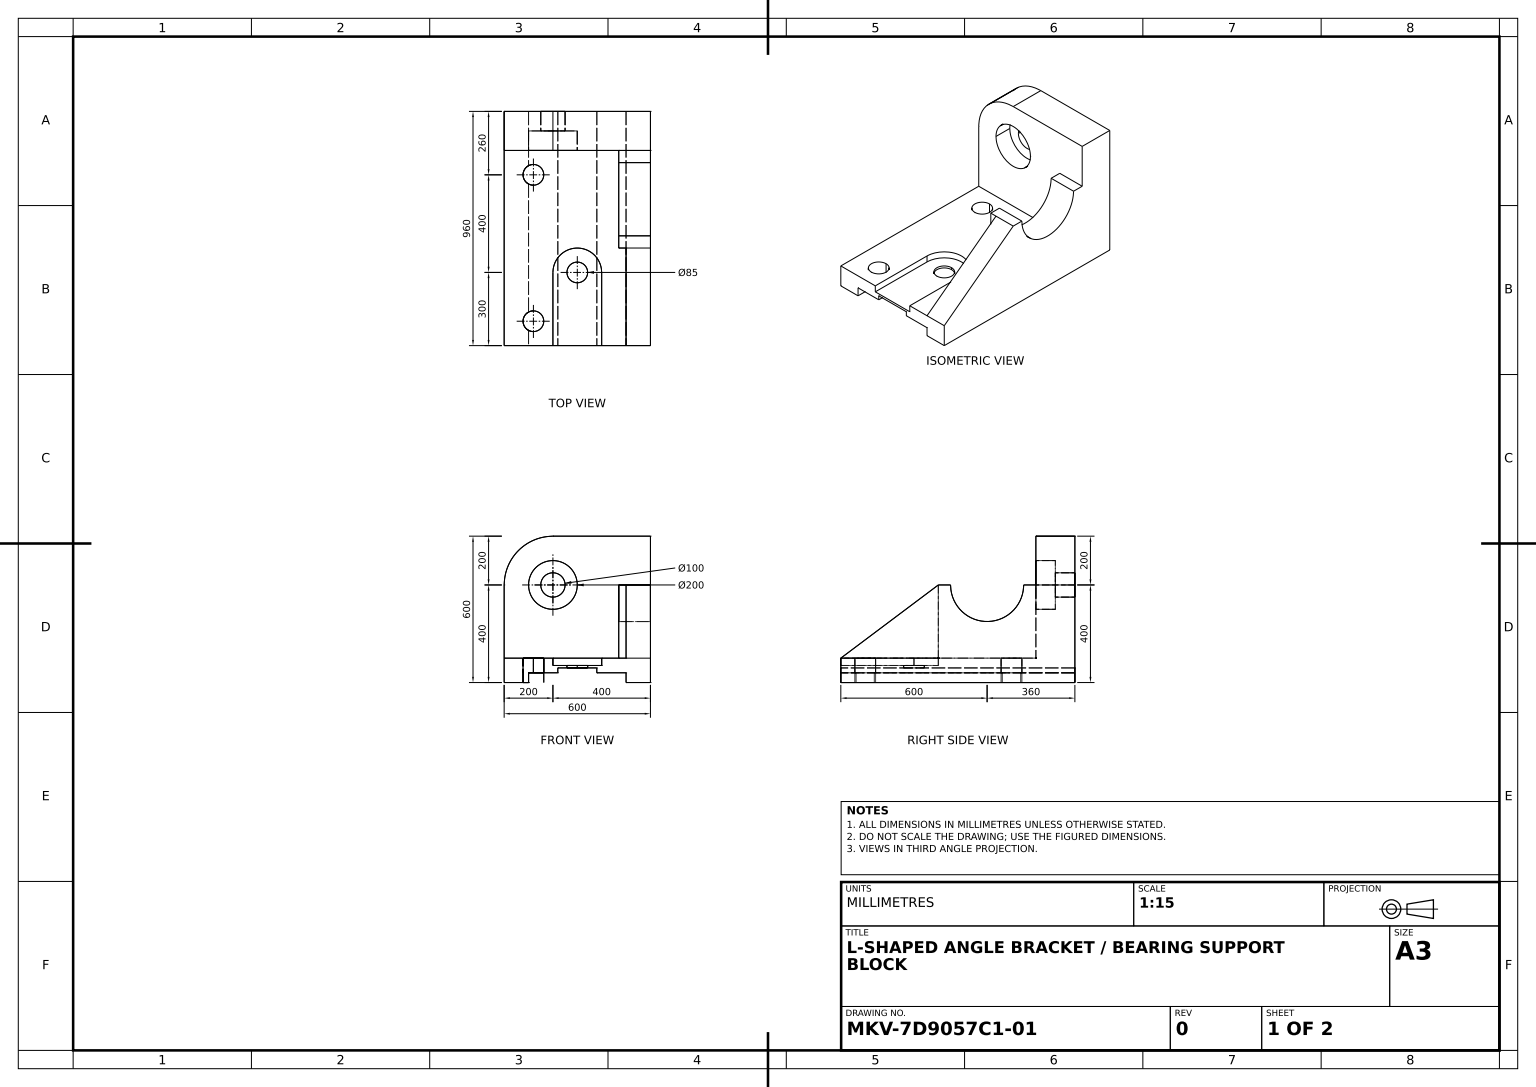
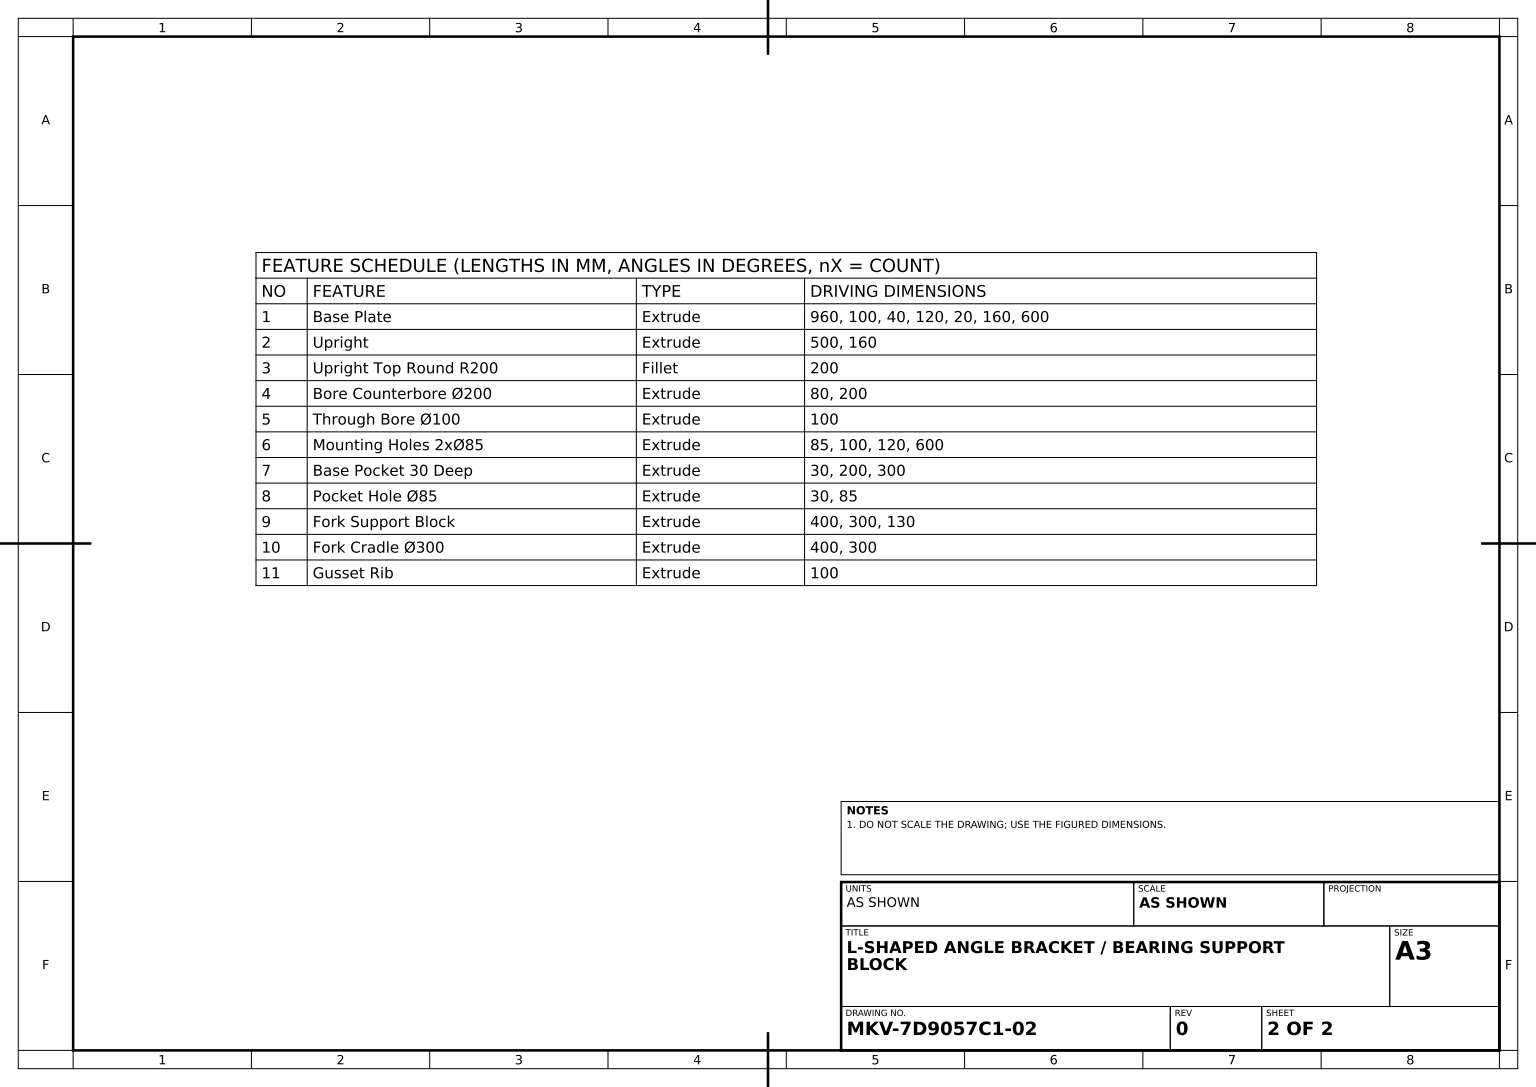
from build123d import *

# Parameters (mm, degrees)
BASE_PLATE_DEPTH            = 960
UPRIGHT_SKETCH_W            = 600
UPRIGHT_SKETCH_H            = 160
UPRIGHT_DEPTH               = 500
UPRIGHT_TOP_ROUND_R200_R    = 200
BORE_COUNTERBORE_SKETCH_R   = 100
BORE_COUNTERBORE_200_DEPTH  = 80
THROUGH_BORE_SKETCH_R       = 50
THROUGH_BORE_100_DEPTH      = 1223.456543195
MOUNTING_HOLES_SKETCH_R     = 42.5
MOUNTING_HOLES_2X_85_DEPTH  = 1238.578280352
BASE_POCKET_30_DEEP_DEPTH   = 30
POCKET_HOLE_SKETCH_R        = 42.5
POCKET_HOLE_85_DEPTH        = 30
FORK_SUPPORT_BLOCK_SKETCH_W = 130
FORK_SUPPORT_BLOCK_SKETCH_H = 300
FORK_SUPPORT_BLOCK_DEPTH    = 400
FORK_CRADLE_SKETCH_R        = 150
FORK_CRADLE_300_DEPTH       = 400
GUSSET_RIB_DEPTH            = 100


with BuildPart() as part:
    # Base Plate Profile Sketch → Base Plate (new body)
    with BuildSketch(Plane.XY):
        Polygon((0, 0), (100, 0), (100, 40), (220, 40), (220, 60), (380, 60), (380, 40), (500, 40), (500, 0), (600, 0), (600, 100), (0, 100), align=None)
    extrude(amount=-BASE_PLATE_DEPTH)

    # Upright Sketch → Upright (add)
    with BuildSketch(Plane(origin=(0, 100, 0), x_dir=(1, 0, 0), z_dir=(0, 1, 0))):
        with Locations((300, 880)):
            Rectangle(UPRIGHT_SKETCH_W, UPRIGHT_SKETCH_H)
    extrude(amount=UPRIGHT_DEPTH)

    # Upright Top Round R200
    upright_top_round_r200_edges = [part.edges().sort_by_distance(p)[0] for p in [
        (0, 600, -880),
    ]]
    fillet(upright_top_round_r200_edges, radius=UPRIGHT_TOP_ROUND_R200_R)

    # Bore Counterbore Sketch → Bore Counterbore Ø200 (cut)
    with BuildSketch(Plane.XY.offset(-800)):
        with Locations((200, 400)):
            Circle(BORE_COUNTERBORE_SKETCH_R)
    extrude(amount=-BORE_COUNTERBORE_200_DEPTH, mode=Mode.SUBTRACT)

    # Through Bore Sketch → Through Bore Ø100 (cut, through all)
    with BuildSketch(Plane.XY.offset(-880)):
        with Locations((200, 400)):
            Circle(THROUGH_BORE_SKETCH_R)
    extrude(amount=-THROUGH_BORE_100_DEPTH, mode=Mode.SUBTRACT)

    # Mounting Holes Sketch → Mounting Holes 2xØ85 (cut, through all)
    with BuildSketch(Plane(origin=(0, 100, 0), x_dir=(1, 0, 0), z_dir=(0, 1, 0))):
        with Locations(Location((120, 700, 0), (0, 0, 270))):
            Circle(MOUNTING_HOLES_SKETCH_R)
        with Locations(Location((120, 100, 0), (0, 0, 270))):
            Circle(MOUNTING_HOLES_SKETCH_R)
    extrude(amount=-MOUNTING_HOLES_2X_85_DEPTH, mode=Mode.SUBTRACT)

    # Base Pocket Sketch → Base Pocket 30 Deep (cut)
    with BuildSketch(Plane(origin=(0, 100, 0), x_dir=(1, 0, 0), z_dir=(0, 1, 0))):
        with BuildLine():
            Line((200, 300), (200, 0))
            Line((200, 0), (400, 0))
            Line((400, 0), (400, 300))
            ThreePointArc((400, 300), (300, 400), (200, 300))
        make_face()
    extrude(amount=-BASE_POCKET_30_DEEP_DEPTH, mode=Mode.SUBTRACT)

    # Pocket Hole Sketch → Pocket Hole Ø85 (cut)
    with BuildSketch(Plane(origin=(0, 70, 0), x_dir=(1, 0, 0), z_dir=(0, 1, 0))):
        with Locations(Location((300, 300, 0), (0, 0, 270))):
            Circle(POCKET_HOLE_SKETCH_R)
    extrude(amount=-POCKET_HOLE_85_DEPTH, mode=Mode.SUBTRACT)

    # Fork Support Block Sketch → Fork Support Block (add)
    with BuildSketch(Plane.XY.offset(-800)):
        with Locations((535, 250)):
            Rectangle(FORK_SUPPORT_BLOCK_SKETCH_W, FORK_SUPPORT_BLOCK_SKETCH_H)
    extrude(amount=FORK_SUPPORT_BLOCK_DEPTH)

    # Fork Cradle Sketch → Fork Cradle Ø300 (cut)
    with BuildSketch(Plane(origin=(600, 0, 0), x_dir=(0, 0, -1), z_dir=(1, 0, 0))):
        with Locations((600, 400)):
            Circle(FORK_CRADLE_SKETCH_R)
    extrude(amount=-FORK_CRADLE_300_DEPTH, mode=Mode.SUBTRACT)

    # Gusset Rib Sketch → Gusset Rib (add)
    with BuildSketch(Plane(origin=(600, 0, 0), x_dir=(0, 0, -1), z_dir=(1, 0, 0))):
        Polygon((400, 400), (400, 100), (0, 100), align=None)
    extrude(amount=-GUSSET_RIB_DEPTH)


solid = part.part
